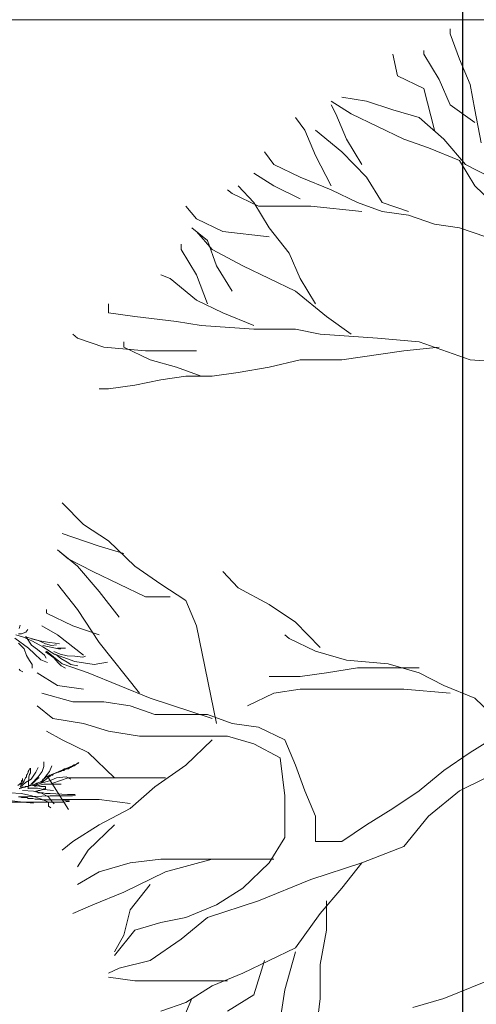
# Model space of a CAD drawing. Units: millimetres. Extents: x 595116 to 630915, y 909473 to 920225.
# Tile 91 of 134: x 629728 to 629744, y 919267 to 919302. Entities that reach past the tile are written whole.
import ezdxf

# ---------------------------------------------------------------- set-up
doc = ezdxf.new("R2010")
doc.units = ezdxf.units.MM
doc.layers.add('Dimension', color=3, linetype='Continuous', lineweight=18)
doc.layers.add('L-PLNT', color=85, linetype='Continuous', lineweight=13)
doc.styles.get("Standard").update_dxf_attribs({"font": 'arial.ttf'})
doc.dimstyles.new('ISO-25', dxfattribs={"dimtxt": 9, "dimasz": 6, "dimexe": 1.25, "dimexo": 0.625, "dimtad": 1, "dimlunit": 4, "dimtxsty": 'Standard', "dimcen": 2.5, "dimadec": 0, "dimazin": 0, "dimtfac": 1, "dimtmove": 0, "dimatfit": 3, "dimfxl": 1, "dimarcsym": 0})

# ---------------------------------------------------------------- blocks, each defined once
blk = doc.blocks.new('A$C4FB75ABC')
for p, q in [((4.5963, 3.4774), (4.6082, 3.5072)), ((4.5657, 3.4153), (4.6395, 3.3917)), ((4.5903, 3.4238), (4.6201, 3.4238)), ((4.6201, 3.4238), (4.6619, 3.4416)), ((4.6619, 3.4416), (4.6798, 3.4655)), ((4.5545, 3.382), (4.6858, 3.2866)), ((4.5903, 3.3343), (4.644, 3.2807)), ((4.6395, 3.3917), (4.7247, 3.3534)), ((4.6551, 3.396), (4.7847, 3.3597)), ((4.6619, 3.3999), (4.7156, 3.3164)), ((4.7156, 3.3761), (4.7931, 3.3582)), ((4.7156, 3.3164), (4.7752, 3.2747)), ((4.7247, 3.3534), (4.8242, 3.2989)), ((4.7847, 3.3597), (4.8521, 3.3286)), ((4.7931, 3.3582), (4.8886, 3.3403)), ((4.8262, 3.3131), (4.9765, 3.282)), ((4.8521, 3.3286), (4.9091, 3.3131)), ((4.8886, 3.3403), (4.9422, 3.3343)), ((4.9091, 3.3131), (4.9558, 3.3183)), ((4.9422, 3.3343), (4.984, 3.3284)), ((4.644, 3.2807), (4.6679, 3.2151)), ((4.6858, 3.2866), (4.7454, 3.233)), ((4.7454, 3.233), (4.8051, 3.1734)), ((4.7752, 3.2747), (4.8408, 3.2211)), ((4.8242, 3.2989), (4.9411, 3.2265)), ((4.8408, 3.2211), (4.8587, 3.1912)), ((4.8521, 3.2509), (4.9299, 3.1939)), ((4.9299, 3.2561), (4.9921, 3.2302)), ((4.9454, 3.2302), (4.9973, 3.1887)), ((4.9454, 3.225), (5.1321, 3.1576)), ((4.9661, 3.2866), (5.0079, 3.2866)), ((4.9765, 3.282), (4.9973, 3.282)), ((4.9921, 3.2302), (5.0595, 3.2146)), ((5.0079, 3.2866), (5.0437, 3.2866)), ((4.6679, 3.2151), (4.6977, 3.1674)), ((4.6977, 3.1674), (4.7215, 3.1316)), ((4.7215, 3.1316), (4.7215, 3.0959)), ((4.8051, 3.1734), (4.8528, 3.1555)), ((4.8528, 3.1555), (4.8707, 3.1495)), ((4.9299, 3.1939), (4.9713, 3.1472)), ((4.9713, 3.1472), (5.0025, 3.1162)), ((4.9973, 3.1887), (5.0595, 3.1524)), ((5.0595, 3.2146), (5.1321, 3.2094)), ((5.0595, 3.1524), (5.0958, 3.1317)), ((5.0958, 3.1317), (5.1632, 3.1162)), ((5.1321, 3.2094), (5.2099, 3.1991)), ((5.1321, 3.1576), (5.3187, 3.1317)), ((5.2099, 3.1991), (5.2358, 3.2094)), ((5.3187, 3.1317), (5.4484, 3.1524)), ((4.5963, 3.0839), (4.6082, 3.072)), ((4.6082, 3.072), (4.6321, 3.0601)), ((5.0025, 3.1162), (5.0439, 3.0954)), ((4.835, 2.1495), (4.835, 2.1952)), ((5.1477, 2.1724), (5.1629, 2.18)), ((5.1553, 2.18), (5.1477, 2.1724)), ((5.1706, 2.1876), (5.1553, 2.18)), ((5.1629, 2.18), (5.1706, 2.1876)), ((4.6749, 2.0733), (4.6825, 2.0961)), ((4.6825, 2.1038), (4.6901, 2.1114)), ((4.6825, 2.0961), (4.6825, 2.1038)), ((4.6901, 2.1114), (4.6977, 2.1266)), ((4.6977, 2.1266), (4.7054, 2.1266)), ((4.7054, 2.0885), (4.6977, 2.0733)), ((4.7054, 2.1266), (4.7054, 2.1343)), ((4.7054, 2.1343), (4.7054, 2.0885)), ((4.713, 2.0275), (4.7587, 2.0961)), ((4.7587, 2.0961), (4.7816, 2.1419)), ((4.7816, 2.0504), (4.8198, 2.1038)), ((4.8121, 2.0047), (4.8884, 2.1038)), ((4.8198, 2.1038), (4.835, 2.1495)), ((4.8884, 2.1038), (4.9113, 2.1571)), ((4.9113, 2.0733), (5.079, 2.1419)), ((4.9113, 2.0733), (4.9265, 2.0809)), ((4.9265, 2.0809), (4.9189, 2.0657)), ((4.9265, 2.0809), (4.957, 2.0885)), ((4.9494, 2.0885), (4.9265, 2.0809)), ((4.9799, 2.1038), (4.9494, 2.0885)), ((4.957, 2.0885), (4.9723, 2.0961)), ((4.9723, 2.0961), (4.9799, 2.0961)), ((5.018, 2.119), (4.9799, 2.1038)), ((4.9799, 2.0961), (4.9952, 2.1038)), ((4.9952, 2.1038), (5.0028, 2.1038)), ((5.0028, 2.1038), (5.0028, 2.1114)), ((5.0028, 2.1114), (5.0257, 2.1114)), ((5.0333, 2.1266), (5.018, 2.119)), ((5.0257, 2.1114), (5.0333, 2.119)), ((5.0562, 2.1343), (5.0333, 2.1266)), ((5.0333, 2.119), (5.0562, 2.1266)), ((5.0714, 2.1419), (5.0562, 2.1343)), ((5.0562, 2.1266), (5.0714, 2.1266)), ((5.1095, 2.1571), (5.0714, 2.1419)), ((5.0714, 2.1266), (5.079, 2.1343)), ((5.079, 2.1343), (5.0867, 2.1419)), ((5.0867, 2.1419), (5.0943, 2.1419)), ((5.0943, 2.1419), (5.1019, 2.1495)), ((5.1019, 2.1495), (5.1095, 2.1495)), ((5.1248, 2.1648), (5.1095, 2.1571)), ((5.1095, 2.1495), (5.1172, 2.1571)), ((5.1172, 2.1571), (5.1248, 2.1571)), ((5.1477, 2.1724), (5.1248, 2.1648)), ((5.1248, 2.1571), (5.1401, 2.1648)), ((5.1401, 2.1648), (5.1477, 2.1724)), ((4.5833, 1.9666), (4.6138, 1.9894)), ((4.6062, 1.9513), (4.6596, 1.9971)), ((4.6138, 1.9894), (4.6215, 2.0047)), ((4.6215, 2.0047), (4.6138, 1.9818)), ((4.6215, 2.0123), (4.6291, 2.0199)), ((4.6215, 2.0047), (4.6215, 2.0123)), ((4.6291, 2.0123), (4.6215, 2.0047)), ((4.6215, 1.9818), (4.6367, 1.9971)), ((4.6291, 2.0199), (4.6291, 2.0352)), ((4.6291, 2.0352), (4.6291, 2.0123)), ((4.6367, 1.9971), (4.6444, 2.0123)), ((4.6444, 2.0123), (4.6596, 2.0428)), ((4.6596, 2.0428), (4.6672, 2.0504)), ((4.6596, 1.9971), (4.713, 2.0275)), ((4.6672, 2.0657), (4.6749, 2.0733)), ((4.6672, 2.0504), (4.6672, 2.0657)), ((4.6901, 2.0504), (4.6825, 1.9361)), ((4.6977, 2.0733), (4.6901, 2.0504)), ((4.713, 1.9818), (4.7816, 2.0504)), ((4.7359, 1.9971), (4.7206, 1.9818)), ((4.7435, 2.0047), (4.7359, 1.9971)), ((4.7511, 2.0123), (4.7435, 2.0047)), ((4.7664, 2.0275), (4.7511, 2.0123)), ((4.7511, 1.9818), (4.7664, 1.9894)), ((4.7511, 1.9666), (4.8045, 1.9894)), ((4.774, 2.0275), (4.7664, 2.0275)), ((4.7664, 1.9894), (4.8045, 2.0047)), ((4.7816, 2.0352), (4.774, 2.0352)), ((4.774, 2.0352), (4.774, 2.0275)), ((4.774, 1.9818), (4.8884, 2.0123)), ((4.7892, 2.0428), (4.7816, 2.0428)), ((4.7816, 2.0428), (4.7816, 2.0352)), ((4.8045, 1.9894), (4.8579, 2.0275)), ((4.8045, 2.0047), (4.8198, 2.0123)), ((4.8198, 2.0123), (4.8274, 2.0275)), ((4.8274, 2.0275), (4.8426, 2.0352)), ((4.8426, 2.0352), (4.8579, 2.0504)), ((4.8579, 2.0275), (4.9113, 2.0733)), ((4.8579, 2.0504), (4.8655, 2.0504)), ((4.8655, 2.0504), (4.8655, 2.058)), ((4.8655, 2.058), (4.8808, 2.058)), ((4.8808, 2.0504), (4.8731, 2.0504)), ((4.8731, 2.0504), (5.0714, 1.7379)), ((4.8808, 2.058), (4.8884, 2.0657)), ((4.896, 2.058), (4.8808, 2.058)), ((4.8808, 2.058), (4.8808, 2.0504)), ((4.8884, 2.0657), (4.9036, 2.0657)), ((4.8884, 2.0123), (4.957, 2.0428)), ((4.9036, 2.0657), (4.896, 2.058)), ((4.9036, 2.0657), (4.9113, 2.0733)), ((4.9189, 2.0657), (4.9036, 2.0657)), ((4.957, 2.0428), (5.0485, 2.0504)), ((5.0485, 2.0504), (5.0943, 2.0275)), ((4.5071, 1.898), (4.6215, 1.8903)), ((4.7725, 1.9851), (4.5975, 1.9398)), ((4.6138, 1.9437), (4.5986, 1.9361)), ((4.6138, 1.9818), (4.6138, 1.9666)), ((4.6138, 1.9742), (4.6215, 1.9818)), ((4.6138, 1.9666), (4.6138, 1.9742)), ((4.6291, 1.9513), (4.6138, 1.9437)), ((4.652, 1.9513), (4.6291, 1.9513)), ((4.6291, 1.9208), (4.7359, 1.9132)), ((4.6596, 1.9589), (4.652, 1.9513)), ((4.6825, 1.9589), (4.6596, 1.9589)), ((4.6901, 1.9666), (4.6825, 1.9589)), ((4.6825, 1.9437), (4.774, 1.9437)), ((4.7054, 1.9742), (4.6901, 1.9666)), ((4.7206, 1.9818), (4.7054, 1.9742)), ((4.7282, 1.9666), (4.7282, 1.9742)), ((4.7282, 1.9742), (4.7359, 1.9742)), ((4.7587, 1.9666), (4.7282, 1.9666)), ((4.7359, 1.9742), (4.7511, 1.9818)), ((4.7359, 1.9132), (4.8045, 1.898)), ((4.7435, 1.9589), (4.835, 1.9818)), ((4.8045, 1.9589), (4.7587, 1.9666)), ((4.7587, 1.9056), (4.7587, 1.9132)), ((4.7587, 1.9132), (4.7664, 1.9132)), ((4.774, 1.9056), (4.7587, 1.9056)), ((4.7664, 1.9132), (4.7816, 1.9208)), ((4.774, 1.9437), (4.835, 1.9285)), ((4.7816, 1.898), (4.774, 1.9056)), ((4.7816, 1.9208), (4.7969, 1.9208)), ((4.8274, 1.898), (4.7816, 1.898)), ((4.7969, 1.9208), (4.8274, 1.9285)), ((4.8503, 1.9589), (4.8045, 1.9589)), ((4.8045, 1.898), (4.8808, 1.8599)), ((4.8274, 1.9285), (4.835, 1.9361)), ((4.8503, 1.8903), (4.8274, 1.898)), ((4.835, 1.9818), (4.9494, 1.9818)), ((4.835, 1.9361), (4.8503, 1.9361)), ((4.835, 1.9285), (4.9265, 1.9208)), ((4.8503, 1.9361), (4.8503, 1.9589)), ((4.9494, 1.9818), (5.0028, 1.9818)), ((4.1639, 1.8065), (5.0333, 1.8065)), ((4.53, 1.8217), (4.6367, 1.8065)), ((4.6062, 1.8599), (4.591, 1.8599)), ((4.591, 1.8599), (4.652, 1.8599)), ((4.6215, 1.8522), (4.6062, 1.8599)), ((4.6215, 1.8903), (4.7206, 1.8675)), ((4.6749, 1.8522), (4.6215, 1.8522)), ((4.6367, 1.8065), (4.7359, 1.7989)), ((4.652, 1.8599), (4.896, 1.8675)), ((4.6825, 1.8446), (4.6749, 1.8522)), ((4.7282, 1.8446), (4.6825, 1.8446)), ((4.7206, 1.8675), (4.8121, 1.837)), ((4.7511, 1.837), (4.7282, 1.8446)), ((4.7816, 1.837), (4.7511, 1.837)), ((4.8198, 1.8294), (4.7816, 1.837)), ((4.8121, 1.837), (4.8808, 1.8065)), ((5.0257, 1.8294), (4.8198, 1.8294)), ((4.896, 1.8903), (4.8503, 1.8903)), ((4.8808, 1.8599), (4.9189, 1.8065)), ((4.8808, 1.8065), (4.8808, 1.7684)), ((5.0638, 1.8827), (4.896, 1.8903)), ((4.896, 1.8675), (5.1095, 1.8675)), ((4.9189, 1.8065), (4.9341, 1.7913)), ((5.0485, 1.8217), (5.0257, 1.8294)), ((5.0333, 1.8065), (5.0562, 1.8141)), ((5.079, 1.8217), (5.0485, 1.8217)), ((5.0562, 1.8141), (5.079, 1.8141)), ((5.1324, 1.8827), (5.0638, 1.8827)), ((5.079, 1.8141), (5.079, 1.8217)), ((5.1095, 1.8675), (5.1248, 1.8751)), ((5.1248, 1.8751), (5.1401, 1.8751)), ((5.1324, 1.8751), (5.1324, 1.8827)), ((5.1401, 1.8751), (5.1324, 1.8751)), ((4.8808, 1.7684), (4.9036, 1.7531))]:
    blk.add_line(p, q)
blk = doc.blocks.new('A$C143125F4')
for p, q in [((1.4606, 4.6814), (1.4606, 4.6994)), ((1.4935, 4.5919), (1.4606, 4.6814)), ((1.2746, 4.5336), (1.2582, 4.6098)), ((1.3676, 4.6098), (1.3676, 4.6232)), ((1.4223, 4.5202), (1.3676, 4.6098)), ((1.5317, 4.5023), (1.4935, 4.5919)), ((1.3676, 4.4888), (1.2746, 4.5336)), ((1.4059, 4.341), (1.3676, 4.4888)), ((1.4606, 4.4306), (1.4223, 4.5202)), ((1.5482, 4.4127), (1.5317, 4.5023)), ((1.0777, 4.4575), (1.1652, 4.444)), ((1.1105, 4.3992), (1.0394, 4.444)), ((1.0558, 4.3992), (1.0394, 4.4306)), ((1.1652, 4.444), (1.2582, 4.4127)), ((1.5482, 4.3679), (1.4606, 4.4306)), ((0.9464, 4.341), (0.9136, 4.3858)), ((1.0941, 4.3096), (1.0558, 4.3992)), ((1.2965, 4.3096), (1.1105, 4.3992)), ((1.2582, 4.4127), (1.3512, 4.3858)), ((1.3512, 4.3858), (1.4387, 4.3096)), ((1.57, 4.2962), (1.5482, 4.4127)), ((0.9847, 4.2514), (0.9464, 4.341)), ((1.0777, 4.2648), (0.9847, 4.341)), ((1.1488, 4.22), (1.0941, 4.3096)), ((1.384, 4.2783), (1.2965, 4.3096)), ((1.4387, 4.3096), (1.5153, 4.22)), ((0.837, 4.22), (0.8042, 4.2648)), ((1.0394, 4.1439), (0.9847, 4.2514)), ((1.1652, 4.1752), (1.0777, 4.2648)), ((1.4935, 4.2335), (1.384, 4.2783)), ((0.93, 4.1752), (0.837, 4.22)), ((1.5482, 4.1439), (1.4935, 4.2335)), ((1.5153, 4.22), (1.6029, 4.1752)), ((0.837, 4.1439), (0.7659, 4.1887)), ((0.7659, 4.0856), (0.7112, 4.1439)), ((0.93, 4.0991), (0.837, 4.1439)), ((1.0394, 4.1304), (0.93, 4.1752)), ((1.2199, 4.0856), (1.1652, 4.1752)), ((1.6412, 4.0543), (1.5482, 4.1439)), ((0.6893, 4.117), (0.6729, 4.1304)), ((0.7823, 4.0722), (0.6893, 4.117)), ((1.1324, 4.0856), (1.0394, 4.1304)), ((0.5635, 4.0274), (0.5252, 4.0722)), ((0.8206, 3.996), (0.7659, 4.0856)), ((0.9683, 4.0722), (0.7823, 4.0722)), ((1.1488, 4.0543), (0.9683, 4.0722)), ((1.2199, 4.0543), (1.1324, 4.0856)), ((1.3129, 4.0543), (1.2199, 4.0856)), ((1.3129, 4.0408), (1.2199, 4.0543)), ((1.4059, 4.0095), (1.3129, 4.0408)), ((0.6565, 3.9826), (0.5635, 4.0274)), ((1.4935, 3.996), (1.4059, 4.0095)), ((0.6018, 3.9512), (0.5471, 3.996)), ((0.6182, 3.9199), (0.5635, 3.9826)), ((0.8206, 3.9647), (0.6565, 3.9826)), ((0.8917, 3.9064), (0.8206, 3.996)), ((1.5865, 3.9647), (1.4935, 3.996)), ((0.5088, 3.9199), (0.5088, 3.9378)), ((0.6346, 3.8616), (0.6018, 3.9512)), ((0.5635, 3.8303), (0.5088, 3.9199)), ((0.7276, 3.8616), (0.6182, 3.9199)), ((0.93, 3.8168), (0.8917, 3.9064)), ((0.4705, 3.8168), (0.4376, 3.8303)), ((0.6018, 3.7272), (0.5635, 3.8303)), ((0.6893, 3.772), (0.6346, 3.8616)), ((0.9136, 3.772), (0.7276, 3.8616)), ((0.5635, 3.7407), (0.4705, 3.8168)), ((0.9847, 3.7272), (0.93, 3.8168)), ((1.023, 3.6824), (0.9136, 3.772)), ((0.2516, 3.6959), (0.2516, 3.7272)), ((0.6565, 3.6959), (0.5635, 3.7407)), ((0.3446, 3.6824), (0.2516, 3.6959)), ((0.7659, 3.6511), (0.6565, 3.6959)), ((0.4923, 3.6645), (0.3446, 3.6824)), ((0.5799, 3.6511), (0.4923, 3.6645)), ((1.1105, 3.6197), (1.023, 3.6824)), ((0.1422, 3.6063), (0.1258, 3.6197)), ((0.7659, 3.6376), (0.5799, 3.6511)), ((0.9136, 3.6376), (0.7659, 3.6376)), ((1.0011, 3.6197), (0.9136, 3.6376)), ((1.2035, 3.6063), (1.0011, 3.6197)), ((0.2352, 3.5749), (0.1422, 3.6063)), ((0.3063, 3.5749), (0.3063, 3.5928)), ((1.3512, 3.5928), (1.2035, 3.6063)), ((1.5317, 3.5301), (1.3512, 3.5928)), ((0.3829, 3.5615), (0.2352, 3.5749)), ((0.3993, 3.5301), (0.3063, 3.5749)), ((0.5635, 3.5615), (0.3829, 3.5615)), ((1.2965, 3.5615), (1.0777, 3.5301)), ((1.4223, 3.5749), (1.2965, 3.5615)), ((0.4923, 3.5032), (0.3993, 3.5301)), ((0.93, 3.5301), (0.8206, 3.5032)), ((1.0777, 3.5301), (0.93, 3.5301)), ((1.6959, 3.5167), (1.5317, 3.5301)), ((0.5799, 3.4719), (0.4923, 3.5032)), ((0.7112, 3.4853), (0.6182, 3.4719)), ((0.8206, 3.5032), (0.7112, 3.4853)), ((0.4376, 3.4584), (0.3446, 3.4405)), ((0.5252, 3.4719), (0.4376, 3.4584)), ((0.6182, 3.4719), (0.5252, 3.4719)), ((0.2516, 3.4271), (0.2188, 3.4271)), ((0.3446, 3.4405), (0.2516, 3.4271)), ((0.1641, 2.9477), (0.0875, 3.0239)), ((0.2516, 2.8895), (0.1641, 2.9477)), ((0.1258, 2.9029), (0.0875, 2.9164)), ((0.2188, 2.8716), (0.1258, 2.9029)), ((0.3446, 2.7999), (0.2516, 2.8895)), ((0.1422, 2.7999), (0.0711, 2.8581)), ((0.1094, 2.8268), (0.0711, 2.8581)), ((0.3063, 2.8447), (0.2188, 2.8716)), ((0.1969, 2.782), (0.1094, 2.8268)), ((0.2188, 2.7103), (0.1422, 2.7999)), ((0.4376, 2.7372), (0.3446, 2.7999)), ((0.3829, 2.6924), (0.1969, 2.782)), ((0.7112, 2.7238), (0.6565, 2.782)), ((0.1422, 2.6476), (0.0711, 2.7372)), ((0.5252, 2.679), (0.4376, 2.7372)), ((0.8206, 2.6655), (0.7112, 2.7238)), ((0.2899, 2.6207), (0.2188, 2.7103)), ((0.4705, 2.6924), (0.3829, 2.6924)), ((0.0328, 2.6342), (0.0328, 2.6476)), ((0.2188, 2.5311), (0.1422, 2.6476)), ((0.5635, 2.5894), (0.5252, 2.679)), ((0.9136, 2.6028), (0.8206, 2.6655)), ((0.1258, 2.5894), (0.0328, 2.6342)), ((0.0711, 2.558), (0.0164, 2.5894)), ((0.2188, 2.558), (0.1258, 2.5894)), ((0.6346, 2.2444), (0.5635, 2.5894)), ((1.0011, 2.5132), (0.9136, 2.6028)), ((0.1641, 2.4863), (0.0711, 2.558)), ((0.8917, 2.5446), (0.8753, 2.558)), ((0.9847, 2.4998), (0.8917, 2.5446)), ((0.3611, 2.3519), (0.2188, 2.5311)), ((0.0875, 2.455), (0.0328, 2.4998)), ((1.0941, 2.4684), (0.9847, 2.4998)), ((0.1805, 2.4236), (0.0875, 2.455)), ((1.1324, 2.4415), (1.023, 2.4236)), ((1.2418, 2.455), (1.0941, 2.4684)), ((1.3512, 2.4415), (1.1324, 2.4415)), ((1.3512, 2.4236), (1.2418, 2.455)), ((0.0711, 2.3788), (0, 2.4236)), ((0.3993, 2.334), (0.1805, 2.4236)), ((0.93, 2.4102), (0.8206, 2.4102)), ((1.023, 2.4236), (0.93, 2.4102)), ((1.4387, 2.3788), (1.3512, 2.4236)), ((0.1641, 2.3654), (0.0711, 2.3788)), ((1.5482, 2.334), (1.4387, 2.3788)), ((0.0164, 2.3519), (0.1258, 2.3206)), ((0.6182, 2.2623), (0.3993, 2.334)), ((0.837, 2.3519), (0.744, 2.3071)), ((0.93, 2.3654), (0.837, 2.3519)), ((1.2965, 2.3654), (0.93, 2.3654)), ((1.4606, 2.3519), (1.2965, 2.3654)), ((1.6412, 2.2444), (1.5482, 2.334)), ((0.0547, 2.2623), (0, 2.3071)), ((0.1258, 2.3206), (0.2352, 2.3206)), ((0.2352, 2.3206), (0.3282, 2.3071)), ((0.3282, 2.3071), (0.4158, 2.2758)), ((0.1641, 2.2444), (0.0547, 2.2623)), ((0.4158, 2.2758), (0.6018, 2.2758)), ((0.6018, 2.2758), (0.6893, 2.2444)), ((0.2516, 2.2175), (0.1641, 2.2444)), ((0.6893, 2.2444), (0.7823, 2.231)), ((0.7823, 2.231), (0.8753, 2.1862)), ((0.0875, 2.1862), (0.0328, 2.2175)), ((0.3611, 2.1996), (0.2516, 2.2175)), ((0.6729, 2.1996), (0.3611, 2.1996)), ((0.7659, 2.1727), (0.6729, 2.1996)), ((1.5317, 2.1414), (1.6247, 2.1996)), ((0.1805, 2.1414), (0.0875, 2.1862)), ((0.6182, 2.1862), (0.5252, 2.0966)), ((0.8589, 2.1235), (0.7659, 2.1727)), ((0.8753, 2.1862), (0.9136, 2.0966)), ((0.2735, 2.0518), (0.1805, 2.1414)), ((0.8753, 1.9891), (0.8589, 2.1235)), ((1.4387, 2.0787), (1.5317, 2.1414)), ((0.5252, 2.0966), (0.4158, 2.0204)), ((0.9136, 2.0966), (0.9464, 2.007)), ((1.3512, 2.007), (1.4387, 2.0787)), ((0.1094, 2.0518), (0.0547, 2.0339)), ((0.4541, 2.0518), (0.1094, 2.0518)), ((0.4158, 2.0204), (0.3282, 1.9443)), ((1.5865, 2.0518), (1.4935, 2.007)), ((0.8753, 1.8412), (0.8753, 1.9891)), ((0.9464, 2.007), (0.9847, 1.9174)), ((1.2582, 1.9443), (1.3512, 2.007)), ((1.4935, 2.007), (1.384, 1.9174)), ((0.2188, 1.9756), (0.0875, 1.9756)), ((0.3282, 1.9622), (0.2188, 1.9756)), ((0.3282, 1.9443), (0.2188, 1.886)), ((0.9847, 1.9174), (0.9847, 1.8278)), ((1.1652, 1.886), (1.2582, 1.9443)), ((1.384, 1.9174), (1.2965, 1.8099)), ((0.2188, 1.886), (0.1258, 1.8278)), ((0.2735, 1.886), (0.1805, 1.7964)), ((1.0777, 1.8278), (1.1652, 1.886)), ((0.1258, 1.8278), (0.0875, 1.7964)), ((0.8206, 1.7516), (0.8753, 1.8412)), ((0.9847, 1.8278), (1.0777, 1.8278)), ((1.2965, 1.8099), (1.1488, 1.7516)), ((0.1805, 1.7964), (0.1422, 1.7382)), ((0.3282, 1.7516), (0.2188, 1.7203)), ((0.4376, 1.7651), (0.3282, 1.7516)), ((0.837, 1.7651), (0.4376, 1.7651)), ((0.6182, 1.7651), (0.4541, 1.7203)), ((0.7276, 1.662), (0.8206, 1.7516)), ((1.1488, 1.7516), (0.9683, 1.6934)), ((1.1488, 1.7516), (1.0777, 1.662)), ((0.2188, 1.7203), (0.1422, 1.6755)), ((0.4541, 1.7203), (0.3063, 1.6486)), ((0.3993, 1.6755), (0.3282, 1.5859)), ((0.9683, 1.6934), (0.7823, 1.6172)), ((0.3063, 1.6486), (0.1969, 1.6038)), ((0.6346, 1.6038), (0.7276, 1.662)), ((1.0777, 1.662), (1.0011, 1.5724)), ((0.1969, 1.6038), (0.1258, 1.5724)), ((0.5252, 1.559), (0.6346, 1.6038)), ((0.7823, 1.6172), (0.6018, 1.559)), ((1.023, 1.6172), (1.023, 1.5142)), ((0.3282, 1.5859), (0.3063, 1.4963)), ((1.0011, 1.5724), (0.9136, 1.4515)), ((0.3446, 1.5142), (0.4376, 1.5411)), ((0.4376, 1.5411), (0.5252, 1.559)), ((0.6018, 1.559), (0.5088, 1.4828)), ((0.2735, 1.4246), (0.3446, 1.5142)), ((0.3063, 1.4963), (0.2735, 1.438)), ((1.023, 1.5142), (1.0011, 1.3932)), ((0.5088, 1.4828), (0.3993, 1.4067)), ((0.9136, 1.4515), (0.7276, 1.3619)), ((0.9136, 1.438), (0.8753, 1.3036)), ((0.3993, 1.4067), (0.2899, 1.3798)), ((0.8042, 1.4067), (0.7659, 1.2857)), ((1.0011, 1.3932), (1.0011, 1.2723)), ((0.2899, 1.3798), (0.2516, 1.3619)), ((0.7276, 1.3619), (0.6182, 1.3171)), ((1.6576, 1.3619), (1.4387, 1.2723)), ((0.3446, 1.335), (0.2516, 1.3484)), ((0.6729, 1.335), (0.3446, 1.335)), ((0.6182, 1.3171), (0.5252, 1.2588)), ((0.8753, 1.3036), (0.8589, 1.1961)), ((0.5252, 1.2588), (0.4376, 1.2275)), ((0.5471, 1.2723), (0.5088, 1.1827)), ((0.7659, 1.2857), (0.6729, 1.2275)), ((1.0011, 1.2723), (0.9847, 1.1379)), ((1.4387, 1.2723), (1.3293, 1.2409))]:
    blk.add_line(p, q)
blk = doc.blocks.new('*D216')
at = {"layer": 'Defpoints', "color": 0, "transparency": 16777216}
for p in [(629505.041, 919411.828), (629743.541, 919411.928), (629743.541, 918832.378)]:
    blk.add_point(p, dxfattribs=at)
at = {"layer": 'Dimension', "color": 0, "lineweight": -2, "transparency": 16777216}
for p, q in [((629505.041, 919411.203), (629505.041, 918831.128)), ((629743.541, 919411.303), (629743.541, 918831.128)), ((629511.041, 918832.378), (629737.541, 918832.378))]:
    blk.add_line(p, q, dxfattribs=at)
at = {"layer": 'Dimension', "color": 0, "transparency": 16777216}
for points in [[(629511.041, 918833.378), (629511.041, 918831.378), (629505.041, 918832.378)], [(629737.541, 918833.378), (629737.541, 918831.378), (629743.541, 918832.378)]]:
    blk.add_solid(points, dxfattribs=at)
at = {"layer": 'Dimension', "color": 0, "transparency": 16777216, "insert": (629624.291, 918837.656), "char_height": 9, "attachment_point": 5}
blk.add_mtext('19\'-10 1/2"', dxfattribs=at)

msp = doc.modelspace()

# ---------------------------------------------------------------- linework, layer by layer
at = {"layer": 'L-PLNT'}
msp.add_line((629824.951, 919302.009), (629511.274, 919302.009), dxfattribs=at)

# ---------------------------------------------------------------- block references
for name, p, xscale, yscale, zscale in [('A$C143125F4', (629728.194, 919253.739), 10.20167662382051, 10.20167662382051, 10.20167662382051), ('A$C4FB75ABC', (629710.284, 919267.014), 3.753413438031968, 3.753413438031968, 3.753413438031968)]:
    msp.add_blockref(name, p, dxfattribs=dict(at, xscale=xscale, yscale=yscale, zscale=zscale))

# ---------------------------------------------------------------- dimensions: what is measured, and where the dimension line sits
at = {"layer": 'Dimension'}
dim = msp.add_linear_dim(base=(629743.541, 918832.378), p1=(629505.041, 919411.828), p2=(629743.541, 919411.928), dimstyle='ISO-25', override={"dimdec": 1, "dimlfac": 1, "dimrnd": 0, "dimzin": 1, "dimdsep": 46, "dimlunit": 4, "dimfrac": 2}, dxfattribs=at)
dim.commit()
dim.dimension.update_dxf_attribs({"geometry": '*D216', "text_midpoint": (629624.291, 918837.656)})

doc.saveas('drawing.dxf')
